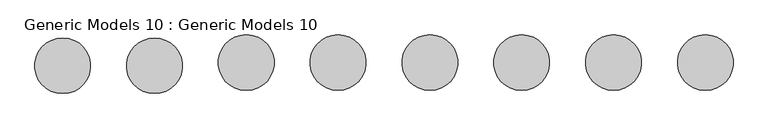
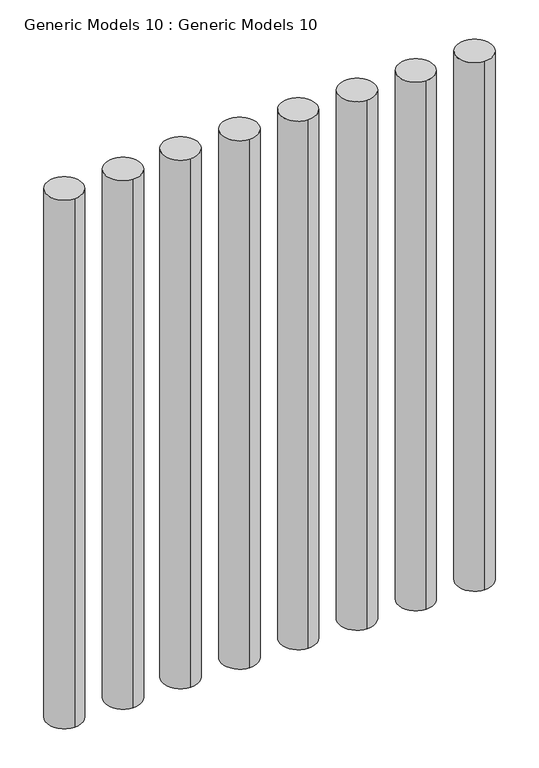
"""IFC4 building model written with IfcOpenShell, lengths in millimetres: proxy geometry, Generic Models 10 : Generic Models 10."""

from ifc_helpers import new_model, si_unit, point, frame, frame_2d, origin, place, context, project, spatial, circle_curve, trimmed, segment, composite_curve, outline, extrude, source, transform, mapped, element, save


def generic_models_10_generic_models_10_d6021447(model_context):
    return source(origin(), model_context, "Body", "SweptSolid", [
        extrude(outline(composite_curve([segment(trimmed(circle_curve(frame_2d((-3754.4136927, -6575.5839066)), 177.8), [point((-3754.4136927, -6753.3839066))], [point((-3754.4136927, -6397.7839066))], False, "CARTESIAN"), True, "CONTINUOUS"), segment(trimmed(circle_curve(frame_2d((-3754.4136927, -6575.5839066)), 177.8), [point((-3754.4136927, -6397.7839066))], [point((-3754.4136927, -6753.3839066))], False, "CARTESIAN"), True, "CONTINUOUS")], self_intersect=False)), frame((0.0, 0.0, 3631.9550828), z_axis=(0.0, 0.0, 1.0), x_axis=(1.0, 0.0, 0.0)), (0.0, 0.0, 1.0), 5551.3034682),
        extrude(outline(composite_curve([segment(trimmed(circle_curve(frame_2d((-3170.2136927, -6575.5839066)), 177.8), [point((-3170.2136927, -6753.3839066))], [point((-3170.2136927, -6397.7839066))], False, "CARTESIAN"), True, "CONTINUOUS"), segment(trimmed(circle_curve(frame_2d((-3170.2136927, -6575.5839066)), 177.8), [point((-3170.2136927, -6397.7839066))], [point((-3170.2136927, -6753.3839066))], False, "CARTESIAN"), True, "CONTINUOUS")], self_intersect=False)), frame((0.0, 0.0, 3631.9550828), z_axis=(0.0, 0.0, 1.0), x_axis=(1.0, 0.0, 0.0)), (0.0, 0.0, 1.0), 5551.3034682),
        extrude(outline(composite_curve([segment(trimmed(circle_curve(frame_2d((-2586.3695716, -6555.1956206)), 177.8), [point((-2586.3695716, -6732.9956206))], [point((-2586.3695716, -6377.3956206))], False, "CARTESIAN"), True, "CONTINUOUS"), segment(trimmed(circle_curve(frame_2d((-2586.3695716, -6555.1956206)), 177.8), [point((-2586.3695716, -6377.3956206))], [point((-2586.3695716, -6732.9956206))], False, "CARTESIAN"), True, "CONTINUOUS")], self_intersect=False)), frame((0.0, 0.0, 3631.9550828), z_axis=(0.0, 0.0, 1.0), x_axis=(1.0, 0.0, 0.0)), (0.0, 0.0, 1.0), 5551.3034682),
        extrude(outline(composite_curve([segment(trimmed(circle_curve(frame_2d((-2002.1695716, -6555.1956206)), 177.8), [point((-2002.1695716, -6732.9956206))], [point((-2002.1695716, -6377.3956206))], False, "CARTESIAN"), True, "CONTINUOUS"), segment(trimmed(circle_curve(frame_2d((-2002.1695716, -6555.1956206)), 177.8), [point((-2002.1695716, -6377.3956206))], [point((-2002.1695716, -6732.9956206))], False, "CARTESIAN"), True, "CONTINUOUS")], self_intersect=False)), frame((0.0, 0.0, 3631.9550828), z_axis=(0.0, 0.0, 1.0), x_axis=(1.0, 0.0, 0.0)), (0.0, 0.0, 1.0), 5551.3034682),
        extrude(outline(composite_curve([segment(trimmed(circle_curve(frame_2d((-1417.9695716, -6555.1956206)), 177.8), [point((-1417.9695716, -6732.9956206))], [point((-1417.9695716, -6377.3956206))], False, "CARTESIAN"), True, "CONTINUOUS"), segment(trimmed(circle_curve(frame_2d((-1417.9695716, -6555.1956206)), 177.8), [point((-1417.9695716, -6377.3956206))], [point((-1417.9695716, -6732.9956206))], False, "CARTESIAN"), True, "CONTINUOUS")], self_intersect=False)), frame((0.0, 0.0, 3631.9550828), z_axis=(0.0, 0.0, 1.0), x_axis=(1.0, 0.0, 0.0)), (0.0, 0.0, 1.0), 5551.3034682),
        extrude(outline(composite_curve([segment(trimmed(circle_curve(frame_2d((-833.7695716, -6555.1956206)), 177.8), [point((-833.7695716, -6732.9956206))], [point((-833.7695716, -6377.3956206))], False, "CARTESIAN"), True, "CONTINUOUS"), segment(trimmed(circle_curve(frame_2d((-833.7695716, -6555.1956206)), 177.8), [point((-833.7695716, -6377.3956206))], [point((-833.7695716, -6732.9956206))], False, "CARTESIAN"), True, "CONTINUOUS")], self_intersect=False)), frame((0.0, 0.0, 3631.9550828), z_axis=(0.0, 0.0, 1.0), x_axis=(1.0, 0.0, 0.0)), (0.0, 0.0, 1.0), 5551.3034682),
        extrude(outline(composite_curve([segment(trimmed(circle_curve(frame_2d((-249.5695716, -6555.1956206)), 177.8), [point((-249.5695716, -6732.9956206))], [point((-249.5695716, -6377.3956206))], False, "CARTESIAN"), True, "CONTINUOUS"), segment(trimmed(circle_curve(frame_2d((-249.5695716, -6555.1956206)), 177.8), [point((-249.5695716, -6377.3956206))], [point((-249.5695716, -6732.9956206))], False, "CARTESIAN"), True, "CONTINUOUS")], self_intersect=False)), frame((0.0, 0.0, 3631.9550828), z_axis=(0.0, 0.0, 1.0), x_axis=(1.0, 0.0, 0.0)), (0.0, 0.0, 1.0), 5551.3034682),
        extrude(outline(composite_curve([segment(trimmed(circle_curve(frame_2d((334.6304284, -6555.1956206)), 177.8), [point((334.6304284, -6732.9956206))], [point((334.6304284, -6377.3956206))], False, "CARTESIAN"), True, "CONTINUOUS"), segment(trimmed(circle_curve(frame_2d((334.6304284, -6555.1956206)), 177.8), [point((334.6304284, -6377.3956206))], [point((334.6304284, -6732.9956206))], False, "CARTESIAN"), True, "CONTINUOUS")], self_intersect=False)), frame((0.0, 0.0, 3631.9550828), z_axis=(0.0, 0.0, 1.0), x_axis=(1.0, 0.0, 0.0)), (0.0, 0.0, 1.0), 5551.3034682),
    ])


if __name__ == "__main__":
    model = new_model("IFC4")
    model_context = context("Model", 3, world=origin())
    ifc_project = project(units=[si_unit("LENGTHUNIT", "METRE", prefix="MILLI")], contexts=[model_context])
    site = spatial("IfcSite", under=ifc_project)
    building = spatial("IfcBuilding", under=site)
    placement = place(None, origin())
    generic_models_10_generic_models_10_shape = generic_models_10_generic_models_10_d6021447(model_context)
    element("IfcBuildingElementProxy", 1, Name="Generic Models 10 : Generic Models 10", ObjectType="Generic Models 10 : Generic Models 10", at=placement, inside=building, context=model_context, shape_type="MappedRepresentation", body=[
        mapped(generic_models_10_generic_models_10_shape, transform((0.0, 0.0, 0.0), x_axis=(1.0, 0.0, 0.0), y_axis=(0.0, 1.0, 0.0), z_axis=(0.0, 0.0, 1.0))),
    ])
    save(model, "model.ifc")

# Revit data of these elements
# Element 1 (IfcBuildingElementProxy, "Generic Models 10 : Generic Models 10")
#   Materials on its faces: "WOODEN SLAT"
# Materials
#   "WOODEN SLAT": class "Generic", colour RGB 120 120 120, transparency 0, Cost = 0
